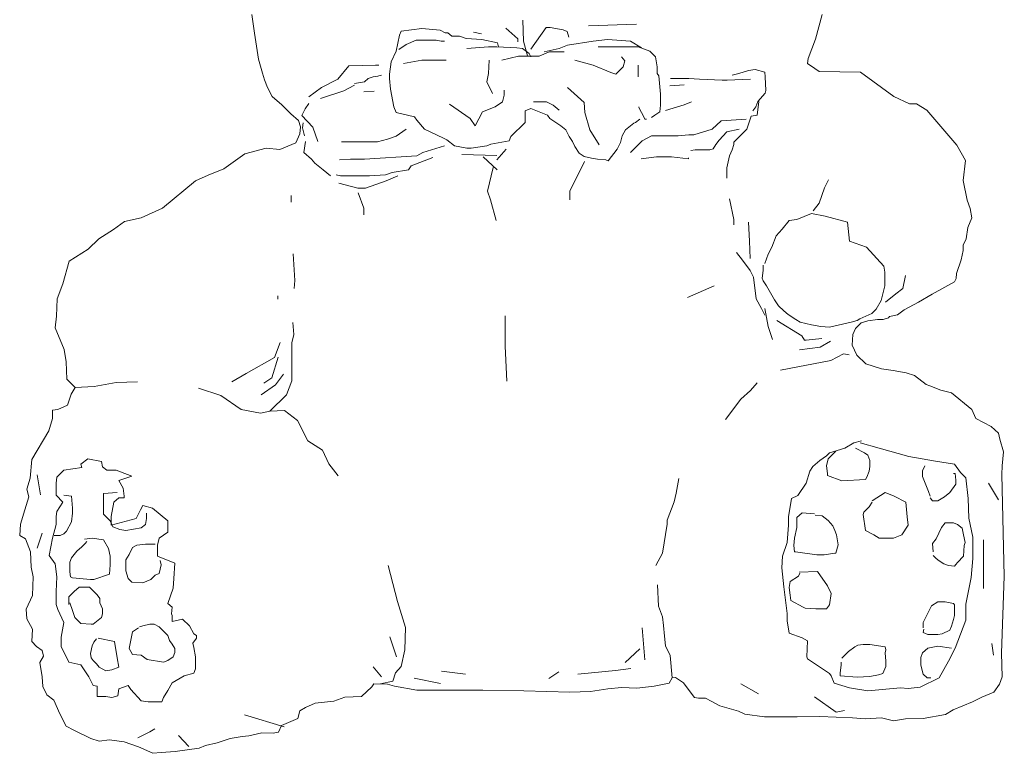
# Model space of a CAD drawing. Units: inches. Extents: x 638 to 1303, y 1 to 699.
# Tile 16 of 21: x 945 to 963, y 577 to 591. Entities that reach past the tile are written whole.
import ezdxf

# ---------------------------------------------------------------- set-up
doc = ezdxf.new("R2010")
doc.units = ezdxf.units.IN
doc.header["$MEASUREMENT"] = 0
doc.layers.add('A-FURN-ACCS', color=8, linetype='Continuous', lineweight=13)

msp = doc.modelspace()

# ---------------------------------------------------------------- linework, layer by layer
at = {"layer": 'A-FURN-ACCS'}
for p, q in [((949.14989, 590.79266), (949.20169, 590.44764)), ((959.42362, 590.34166), (959.54608, 590.79084)), ((951.8738, 590.48873), (952.25259, 590.53415)), ((952.25259, 590.53415), (952.58592, 590.50387)), ((953.77913, 590.53989), (953.99984, 590.34875)), ((954.08812, 590.68691), (954.10284, 590.30464)), ((954.23526, 590.15762), (954.51482, 590.55459)), ((954.51482, 590.55459), (954.58839, 590.55459)), ((954.58839, 590.55459), (954.82381, 590.51048)), ((955.28684, 590.58509), (956.16525, 590.61435)), ((949.20169, 590.44764), (949.27456, 589.97731)), ((951.7829, 590.12537), (951.84351, 590.41303)), ((951.84351, 590.41303), (951.8738, 590.48873)), ((952.58592, 590.50387), (952.67683, 590.45845)), ((952.67683, 590.45845), (952.72227, 590.45845)), ((952.72227, 590.45845), (952.79803, 590.39789)), ((952.79803, 590.39789), (952.93439, 590.39789)), ((952.93439, 590.39789), (953.05561, 590.35247)), ((953.05561, 590.35247), (953.34348, 590.33733)), ((953.19059, 590.46637), (953.33772, 590.43697)), ((953.99984, 590.34875), (953.99984, 590.28994)), ((954.82381, 590.51048), (954.89738, 590.48107)), ((954.89738, 590.48107), (954.92681, 590.37816)), ((951.82835, 590.15565), (951.96471, 590.24649)), ((951.96471, 590.24649), (952.14653, 590.32219)), ((952.14653, 590.32219), (952.51016, 590.32219)), ((952.51016, 590.32219), (952.60107, 590.30705)), ((952.60107, 590.30705), (952.66167, 590.30705)), ((953.07076, 590.17079), (953.46469, 590.20107)), ((953.34348, 590.33733), (953.63136, 590.27677)), ((953.46469, 590.20107), (953.61621, 590.20107)), ((953.61621, 590.20107), (953.97984, 590.18593)), ((953.63136, 590.27677), (953.6465, 590.20107)), ((953.97984, 590.18593), (954.0859, 590.17079)), ((954.0859, 590.17079), (954.2071, 590.07995)), ((954.10284, 590.30464), (954.17641, 590.04)), ((954.47983, 590.11023), (954.75255, 590.17079)), ((954.75255, 590.17079), (954.90406, 590.23135)), ((954.90406, 590.23135), (955.37375, 590.30705)), ((955.37375, 590.30705), (955.63132, 590.33733)), ((955.46466, 590.20107), (956.19192, 590.20107)), ((955.63132, 590.33733), (956.05556, 590.30705)), ((956.05556, 590.30705), (956.25253, 590.18593)), ((956.19192, 590.20107), (956.40404, 590.12537)), ((959.29283, 589.9888), (959.42362, 590.34166)), ((951.69199, 589.92855), (951.7829, 590.12537)), ((953.70711, 589.95883), (954.01014, 590.03453)), ((954.01014, 590.03453), (954.38892, 590.03453)), ((954.2071, 590.07995), (954.2374, 590.01939)), ((954.38892, 590.03453), (954.57073, 590.11023)), ((954.57073, 590.11023), (954.84346, 590.11023)), ((955.9495, 589.94369), (955.8889, 590.01939)), ((956.40404, 590.12537), (956.5101, 590.01939)), ((956.5101, 590.01939), (956.5404, 589.83771)), ((959.27975, 589.89732), (959.29283, 589.9888)), ((949.27456, 589.97731), (949.30982, 589.84812)), ((949.30982, 589.84812), (949.34508, 589.71893)), ((950.72231, 589.61062), (950.91928, 589.85285)), ((950.91928, 589.85285), (951.40411, 589.86799)), ((951.40411, 589.86799), (951.46472, 589.86799)), ((951.66169, 589.70145), (951.69199, 589.92855)), ((951.91926, 589.89827), (952.25259, 589.95883)), ((952.25259, 589.95883), (952.38895, 589.95883)), ((952.38895, 589.95883), (952.61622, 589.95883)), ((952.61622, 589.95883), (952.69198, 589.95883)), ((953.47984, 589.95883), (953.46469, 589.71659)), ((955.04042, 589.95883), (955.37375, 589.86799)), ((955.37375, 589.86799), (955.69193, 589.73173)), ((955.78284, 589.70145), (955.9192, 589.83771)), ((955.9192, 589.83771), (955.9495, 589.94369)), ((956.19192, 589.86799), (956.19192, 589.65603)), ((956.5404, 589.83771), (956.5404, 589.71659)), ((959.41054, 589.80584), (959.27975, 589.89732)), ((959.48901, 589.75356), (959.41054, 589.80584)), ((949.34508, 589.71893), (949.38034, 589.60149)), ((951.2085, 589.56653), (951.27306, 589.62746)), ((951.27306, 589.62746), (951.36274, 589.65255)), ((951.36274, 589.65255), (951.44882, 589.66689)), ((951.44882, 589.66689), (951.46676, 589.67047)), ((951.46676, 589.67047), (951.51338, 589.68839)), ((951.66169, 589.62575), (951.66169, 589.70145)), ((951.67684, 589.42893), (951.66169, 589.62575)), ((953.46469, 589.71659), (953.43439, 589.56519)), ((955.69193, 589.73173), (955.78284, 589.70145)), ((956.5404, 589.71659), (956.5707, 589.67117)), ((956.5707, 589.67117), (956.60101, 589.3381)), ((956.78282, 589.62575), (957.11615, 589.62575)), ((957.11615, 589.62575), (957.31312, 589.61062)), ((957.90322, 589.6858), (958.02658, 589.71661)), ((958.02658, 589.71661), (958.20132, 589.76797)), ((958.20132, 589.76797), (958.32467, 589.78852)), ((958.32467, 589.78852), (958.49942, 589.73716)), ((958.49942, 589.73716), (958.5097, 589.65499)), ((958.5097, 589.65499), (958.51998, 589.40847)), ((960.24757, 589.74049), (959.48901, 589.75356)), ((960.84919, 589.29615), (960.24757, 589.74049)), ((949.38034, 589.60149), (949.4391, 589.46056)), ((949.4391, 589.46056), (949.52138, 589.29614)), ((950.19201, 589.29267), (950.41928, 589.45922)), ((950.41928, 589.45922), (950.72231, 589.61062)), ((950.82837, 589.39866), (951.02533, 589.50463)), ((951.02556, 589.53427), (951.2085, 589.56653)), ((953.43439, 589.56519), (953.54045, 589.35323)), ((954.90406, 589.45922), (955.20709, 589.1867)), ((956.77251, 589.49064), (957.02949, 589.51119)), ((957.31312, 589.61062), (957.7222, 589.59547)), ((957.7222, 589.59547), (957.81311, 589.59547)), ((957.81311, 589.59547), (958.23734, 589.61062)), ((949.52138, 589.29614), (949.69767, 589.14347)), ((950.40413, 589.2624), (950.82837, 589.39866)), ((951.19173, 589.38237), (951.38125, 589.39351)), ((951.73744, 589.111), (951.67684, 589.42893)), ((953.72226, 589.20184), (953.75256, 589.32296)), ((953.75256, 589.32296), (953.75256, 589.4138)), ((956.60101, 589.3381), (956.60101, 589.14128)), ((958.5097, 589.35711), (958.37606, 589.20304)), ((958.51998, 589.40847), (958.5097, 589.35711)), ((961.13692, 589.16547), (960.84919, 589.29615)), ((949.69767, 589.14347), (949.86221, 588.97905)), ((950.18839, 589.17071), (950.1215, 589.07045)), ((951.7829, 589.00502), (951.73744, 589.111)), ((952.75258, 589.15642), (953.13136, 588.89904)), ((953.35863, 589.02016), (953.5859, 589.111)), ((953.5859, 589.111), (953.72226, 589.20184)), ((954.28286, 589.20184), (954.52528, 589.20184)), ((954.52528, 589.20184), (954.64649, 589.14128)), ((954.64649, 589.14128), (954.75255, 589.05044)), ((955.20709, 589.1867), (955.22224, 589.00502)), ((956.20707, 589.09586), (956.20707, 589.111)), ((956.25253, 589.00502), (956.20707, 589.09586)), ((956.60101, 589.14128), (956.58586, 589.02016)), ((956.69168, 589.0428), (957.03133, 589.14723)), ((957.03133, 589.14723), (957.16197, 589.19944)), ((958.33495, 589.11059), (958.28356, 589.0387)), ((958.37606, 589.20304), (958.33495, 589.11059)), ((958.39184, 589.20497), (958.36043, 588.95382)), ((961.2677, 589.16547), (961.13692, 589.16547)), ((961.4508, 589.04785), (961.2677, 589.16547)), ((949.86221, 588.97905), (950.00324, 588.86161)), ((950.1215, 589.07045), (950.06575, 588.94792)), ((950.06575, 588.94792), (950.26642, 588.73626)), ((952.11623, 588.92932), (951.7829, 589.00502)), ((952.16168, 588.86876), (952.11623, 588.92932)), ((953.22227, 588.76278), (953.35863, 589.02016)), ((954.2374, 589.08072), (954.13134, 589.0353)), ((954.13134, 589.0353), (954.13134, 588.91418)), ((954.13134, 588.91418), (954.13134, 588.82334)), ((954.54043, 588.9596), (954.2374, 589.08072)), ((954.58588, 588.89904), (954.54043, 588.9596)), ((955.22224, 589.00502), (955.31315, 588.68708)), ((956.29798, 588.92932), (956.25253, 589.00502)), ((956.31313, 588.8839), (956.29798, 588.92932)), ((956.49495, 588.9596), (956.43434, 588.91418)), ((956.58586, 589.02016), (956.49495, 588.9596)), ((958.25047, 588.93813), (958.17192, 588.70267)), ((958.36043, 588.95382), (958.25047, 588.93813)), ((962.00011, 588.40748), (961.4508, 589.04785)), ((950.00324, 588.86161), (950.03851, 588.74417)), ((950.03851, 588.74417), (950.02675, 588.61498)), ((950.08805, 588.81424), (950.0769, 588.72511)), ((950.26642, 588.73626), (950.35561, 588.48004)), ((952.29804, 588.70222), (952.16168, 588.86876)), ((953.13136, 588.89904), (953.22227, 588.76278)), ((954.13134, 588.82334), (953.87378, 588.56596)), ((954.78285, 588.76278), (954.58588, 588.89904)), ((954.87376, 588.68708), (954.78285, 588.76278)), ((956.11617, 588.8082), (955.96465, 588.68708)), ((956.14647, 588.82334), (956.11617, 588.8082)), ((956.22223, 588.8839), (956.14647, 588.82334)), ((956.34344, 588.8839), (956.31313, 588.8839)), ((957.54039, 588.70222), (957.70705, 588.85362)), ((957.70705, 588.85362), (958.16159, 588.8839)), ((950.02675, 588.61498), (949.95623, 588.45056)), ((950.0769, 588.72511), (950.11035, 588.5803)), ((951.62302, 588.52065), (951.77978, 588.57286)), ((951.77978, 588.57286), (951.96268, 588.7034)), ((952.64652, 588.53568), (952.29804, 588.70222)), ((953.87378, 588.56596), (953.84347, 588.49026)), ((954.93437, 588.56596), (954.87376, 588.68708)), ((954.99497, 588.47512), (954.93437, 588.56596)), ((955.31315, 588.68708), (955.47981, 588.41456)), ((955.90404, 588.5811), (955.87375, 588.45998)), ((955.96465, 588.68708), (955.90404, 588.5811)), ((956.26768, 588.49026), (956.43434, 588.5811)), ((956.43434, 588.5811), (956.91918, 588.5811)), ((956.91918, 588.5811), (957.11615, 588.59624)), ((957.11615, 588.59624), (957.20706, 588.59624)), ((957.20706, 588.59624), (957.54039, 588.70222)), ((957.81063, 588.65558), (957.66925, 588.49862)), ((958.03054, 588.70267), (957.81063, 588.65558)), ((958.17192, 588.70267), (957.93629, 588.46722)), ((949.95623, 588.45056), (949.66241, 588.33312)), ((950.13141, 588.47512), (950.1011, 588.2783)), ((950.78695, 588.46843), (951.44013, 588.46843)), ((951.44013, 588.46843), (951.62302, 588.52065)), ((952.66167, 588.39942), (952.26774, 588.2783)), ((952.70713, 588.5054), (952.64652, 588.53568)), ((952.84349, 588.39942), (952.70713, 588.5054)), ((953.07076, 588.354), (952.84349, 588.39942)), ((953.43439, 588.39942), (953.14652, 588.354)), ((953.51015, 588.4297), (953.43439, 588.39942)), ((953.84347, 588.49026), (953.51015, 588.4297)), ((955.04042, 588.38428), (954.99497, 588.47512)), ((955.11618, 588.26316), (955.04042, 588.38428)), ((955.87375, 588.45998), (955.81314, 588.33886)), ((956.05556, 588.2783), (956.26768, 588.49026)), ((957.60641, 588.42013), (957.55929, 588.34165)), ((957.66925, 588.49862), (957.60641, 588.42013)), ((957.93629, 588.42013), (957.90488, 588.32595)), ((957.93629, 588.46722), (957.93629, 588.42013)), ((962.15705, 588.13303), (962.00011, 588.40748)), ((949.02775, 588.25091), (948.6399, 587.98079)), ((949.4156, 588.35661), (949.02775, 588.25091)), ((949.66241, 588.33312), (949.4156, 588.35661)), ((950.1011, 588.2783), (950.23747, 588.15718)), ((952.16168, 588.21774), (951.20715, 588.15718)), ((952.26774, 588.2783), (952.16168, 588.21774)), ((952.98128, 588.24184), (953.61533, 588.22036)), ((953.14652, 588.354), (953.07076, 588.354)), ((953.36816, 588.19888), (953.62608, 587.96263)), ((953.61533, 588.14519), (953.78729, 588.33849)), ((955.20709, 588.2026), (955.11618, 588.26316)), ((955.34345, 588.17232), (955.20709, 588.2026)), ((955.81314, 588.33886), (955.64648, 588.1269)), ((956.24855, 588.16053), (956.52467, 588.19502)), ((956.52467, 588.19502), (956.80081, 588.19502)), ((956.80081, 588.19502), (957.11145, 588.16053)), ((957.22941, 588.32595), (957.15086, 588.31025)), ((957.49645, 588.32595), (957.22941, 588.32595)), ((957.55929, 588.34165), (957.49645, 588.32595)), ((957.85775, 588.21608), (957.81063, 587.99632)), ((957.90488, 588.32595), (957.85775, 588.21608)), ((950.23747, 588.15718), (950.29807, 588.08148)), ((950.29807, 588.08148), (950.44959, 587.96036)), ((950.94957, 588.15718), (950.75261, 588.14204)), ((951.20715, 588.15718), (950.94957, 588.15718)), ((952.05562, 588.03606), (952.01017, 587.96036)), ((952.44955, 588.18746), (952.05562, 588.03606)), ((955.21288, 588.11011), (954.94507, 587.5749)), ((955.44951, 588.15718), (955.34345, 588.17232)), ((955.60102, 588.14204), (955.44951, 588.15718)), ((955.64648, 588.1269), (955.60102, 588.14204)), ((957.11145, 588.16053), (957.11145, 588.17778)), ((962.11781, 587.7671), (962.15705, 588.13303)), ((948.35783, 587.86335), (948.12277, 587.75766)), ((948.6399, 587.98079), (948.35783, 587.86335)), ((950.44959, 587.96036), (950.58594, 587.85438)), ((950.76776, 587.85438), (950.692, 587.86952)), ((951.29806, 587.85438), (950.76776, 587.85438)), ((951.58593, 587.86952), (951.29806, 587.85438)), ((951.70714, 587.91494), (951.58593, 587.86952)), ((951.60108, 587.76354), (951.8132, 587.85438)), ((952.01017, 587.96036), (951.70714, 587.91494)), ((953.5525, 588.00307), (953.44538, 587.5749)), ((957.81063, 587.99632), (957.81063, 587.80796)), ((948.12277, 587.75766), (947.52337, 587.2644)), ((950.73746, 587.71812), (951.08594, 587.62728)), ((951.2223, 587.62728), (951.60108, 587.76354)), ((959.66424, 587.77656), (959.5857, 587.63529)), ((962.18884, 587.41007), (962.11781, 587.7671)), ((949.87061, 587.49189), (949.87061, 587.3701)), ((951.08594, 587.62728), (951.2223, 587.62728)), ((951.08837, 587.53971), (951.19192, 587.26378)), ((953.44538, 587.5749), (953.49894, 587.41434)), ((954.94507, 587.5749), (954.94507, 587.41434)), ((959.5857, 587.63529), (959.49144, 587.35275)), ((953.49894, 587.41434), (953.60607, 587.0397)), ((957.85775, 587.43123), (957.93629, 587.05451)), ((959.49144, 587.35275), (959.38149, 587.21148)), ((962.2442, 587.25794), (962.18884, 587.41007)), ((947.52337, 587.2644), (947.13552, 587.08824)), ((951.19192, 587.26378), (951.19192, 587.14306)), ((959.08302, 587.05451), (959.35007, 587.16439)), ((959.35007, 587.16439), (959.6014, 587.1173)), ((959.6014, 587.1173), (960.00983, 587.00742)), ((962.27188, 587.08507), (962.2442, 587.25794)), ((946.82995, 587.01777), (946.63014, 586.87684)), ((947.13552, 587.08824), (946.82995, 587.01777)), ((957.93629, 587.05451), (957.93629, 586.96033)), ((958.20334, 587.00742), (958.21905, 586.66209)), ((958.81597, 586.88184), (958.94165, 587.03881)), ((958.94165, 587.03881), (959.08302, 587.05451)), ((960.00983, 587.00742), (960.04124, 586.66209)), ((962.20268, 586.9122), (962.27188, 587.08507)), ((946.63014, 586.87684), (946.36692, 586.7061)), ((958.62747, 586.55221), (958.70601, 586.75627)), ((958.70601, 586.75627), (958.81597, 586.88184)), ((962.16808, 586.70477), (962.20268, 586.9122)), ((946.36692, 586.7061), (946.16711, 586.51819)), ((958.21905, 586.66209), (958.23476, 586.34815)), ((960.04124, 586.66209), (960.35542, 586.55221)), ((962.11272, 586.58721), (962.16808, 586.70477)), ((962.11272, 586.49041), (962.11272, 586.58721)), ((946.16711, 586.51819), (945.82628, 586.29505)), ((949.90596, 586.42933), (949.93844, 585.94243)), ((957.98342, 586.45803), (958.09338, 586.31676)), ((958.50181, 586.25397), (958.56464, 586.42664)), ((958.56464, 586.42664), (958.62747, 586.55221)), ((960.35542, 586.55221), (960.66959, 586.20688)), ((962.07812, 586.32445), (962.11272, 586.49041)), ((945.82628, 586.29505), (945.70875, 585.88401)), ((958.09338, 586.31676), (958.23476, 586.1284)), ((958.47038, 586.1284), (958.47038, 586.22258)), ((961.99508, 586.07552), (962.07812, 586.32445)), ((958.23476, 586.1284), (958.29759, 586.00282)), ((958.45468, 585.98713), (958.47038, 586.1284)), ((960.66959, 586.20688), (960.6853, 586.097)), ((960.6853, 586.097), (960.6853, 585.84586)), ((961.98816, 585.97872), (961.99508, 586.07552)), ((945.70875, 585.88401), (945.60297, 585.61389)), ((949.93844, 585.94243), (949.9222, 585.79636)), ((958.29759, 586.00282), (958.34472, 585.6104)), ((958.47038, 585.94004), (958.45468, 585.98713)), ((958.53322, 585.84586), (958.47038, 585.94004)), ((961.0623, 586.03422), (961.01518, 585.79876)), ((961.55004, 585.69846), (961.96048, 585.9234)), ((961.96048, 585.9234), (961.98816, 585.97872)), ((957.57905, 585.84784), (957.09156, 585.63472)), ((958.6746, 585.59471), (958.53322, 585.84586)), ((960.6853, 585.84586), (960.62246, 585.57901)), ((960.88951, 585.70458), (960.70101, 585.54762)), ((961.01518, 585.79876), (960.88951, 585.70458)), ((961.30092, 585.55325), (961.55004, 585.69846)), ((945.60297, 585.61389), (945.59122, 585.2968)), ((949.62687, 585.66517), (949.62687, 585.60428)), ((958.34472, 585.6104), (958.43897, 585.43774)), ((958.75314, 585.48483), (958.6746, 585.59471)), ((960.62246, 585.57901), (960.52821, 585.42204)), ((961.03796, 585.40804), (961.30092, 585.55325)), ((958.43897, 585.43774), (958.50181, 585.31216)), ((958.50181, 585.43774), (958.56464, 585.1081)), ((958.84739, 585.39065), (958.75314, 585.48483)), ((958.92593, 585.32786), (958.84739, 585.39065)), ((959.06731, 585.23368), (958.92593, 585.32786)), ((960.44967, 585.34356), (960.22975, 585.24938)), ((960.52821, 585.42204), (960.44967, 585.34356)), ((960.92032, 585.31815), (961.03796, 585.40804)), ((945.59122, 585.2968), (945.56771, 585.0854)), ((949.91721, 584.95945), (949.90037, 585.17828)), ((953.77053, 585.29983), (953.77053, 584.75181)), ((958.72172, 585.21798), (959.17727, 584.93544)), ((959.14586, 585.18659), (959.06731, 585.23368)), ((959.35007, 585.1395), (959.14586, 585.18659)), ((960.07266, 585.18659), (959.67995, 585.09241)), ((960.18262, 585.21798), (960.07266, 585.18659)), ((960.15222, 585.06922), (960.25601, 585.17294)), ((960.22975, 585.24938), (960.18262, 585.21798)), ((960.25601, 585.17294), (960.38057, 585.20752)), ((960.38057, 585.20752), (960.55357, 585.23517)), ((960.55357, 585.23517), (960.65737, 585.23517)), ((960.65737, 585.23517), (960.75424, 585.26283)), ((960.75424, 585.26283), (960.77501, 585.29049)), ((960.77501, 585.29049), (960.92032, 585.31815)), ((945.56771, 585.0854), (945.73225, 584.6861)), ((958.56464, 585.1081), (958.64318, 584.87265)), ((959.52286, 585.1081), (959.35007, 585.1395)), ((959.67995, 585.09241), (959.52286, 585.1081)), ((960.10377, 584.95859), (960.15222, 585.06922)), ((949.67082, 584.81513), (949.56443, 584.54176)), ((949.88352, 584.80795), (949.91721, 584.95945)), ((949.88352, 584.40396), (949.88352, 584.80795)), ((959.17727, 584.93544), (959.2244, 584.85695)), ((959.2244, 584.85695), (959.25581, 584.85695)), ((959.25581, 584.85695), (959.53857, 584.88835)), ((959.50715, 584.73138), (959.69565, 584.84126)), ((960.08993, 584.76498), (960.10377, 584.95859)), ((945.73225, 584.6861), (945.76751, 584.46296)), ((953.77053, 584.75181), (953.801, 584.11246)), ((959.13015, 584.68429), (959.50715, 584.73138)), ((959.70471, 584.48715), (959.93399, 584.61052)), ((959.93399, 584.61052), (960.03981, 584.5929)), ((960.1799, 584.58519), (960.08993, 584.76498)), ((945.76751, 584.46296), (945.77926, 584.14587)), ((949.56443, 584.54176), (949.04768, 584.25321)), ((949.62984, 584.54666), (949.51615, 584.17338)), ((958.78756, 584.31091), (959.70471, 584.48715)), ((960.33905, 584.42615), (960.1799, 584.58519)), ((960.62969, 584.33626), (960.33905, 584.42615)), ((949.04768, 584.25321), (948.78931, 584.10134)), ((949.88352, 584.25246), (949.88352, 584.40396)), ((949.88352, 584.1178), (949.88352, 584.25246)), ((960.83729, 584.3086), (960.62969, 584.33626)), ((961.07948, 584.2602), (960.83729, 584.3086)), ((961.23172, 584.2118), (961.07948, 584.2602)), ((945.77926, 584.14587), (945.93205, 583.99319)), ((946.27853, 584.0168), (946.68283, 584.08413)), ((946.68283, 584.08413), (947.07028, 584.10097)), ((949.51615, 584.17338), (949.36997, 584.076)), ((949.72729, 584.2383), (949.58111, 584.04354)), ((949.78245, 583.8653), (949.88352, 584.1178)), ((958.24081, 583.9408), (958.36426, 584.0818)), ((961.43931, 584.05276), (961.23172, 584.2118)), ((945.93205, 583.99319), (945.86154, 583.87576)), ((945.93205, 583.99319), (946.27853, 584.0168)), ((948.18211, 583.98313), (948.5864, 583.84847)), ((949.58111, 584.04354), (949.32124, 583.86501)), ((958.06443, 583.78218), (958.24081, 583.9408)), ((961.50851, 584.0251), (961.43931, 584.05276)), ((961.70919, 583.94904), (961.50851, 584.0251)), ((961.90295, 583.90064), (961.70919, 583.94904)), ((962.27066, 583.59232), (961.90295, 583.90064)), ((945.86154, 583.87576), (945.79102, 583.6761)), ((948.5864, 583.84847), (948.95701, 583.59597)), ((949.47922, 583.5623), (949.78245, 583.8653)), ((957.78223, 583.41208), (958.06443, 583.78218)), ((945.61472, 583.59389), (945.5207, 583.58215)), ((945.5207, 583.58215), (945.5207, 583.42947)), ((945.79102, 583.6761), (945.61472, 583.59389)), ((948.95701, 583.59597), (949.31077, 583.52864)), ((949.31077, 583.52864), (949.47922, 583.5623)), ((949.47922, 583.5623), (949.74876, 583.57914)), ((949.74876, 583.57914), (949.9846, 583.39397)), ((962.34678, 583.43329), (962.27066, 583.59232)), ((945.5207, 583.42947), (945.45018, 583.20634)), ((949.9846, 583.39397), (950.1699, 583.02364)), ((962.62358, 583.28808), (962.34678, 583.43329)), ((945.45018, 583.20634), (945.14507, 582.68286)), ((962.76198, 583.16361), (962.62358, 583.28808)), ((950.1699, 583.02364), (950.43943, 582.85532)), ((960.12587, 582.98582), (960.26454, 583.02739)), ((962.78273, 583.05298), (962.76198, 583.16361)), ((962.85194, 582.82479), (962.78273, 583.05298)), ((950.43943, 582.85532), (950.55735, 582.60282)), ((959.65441, 582.69484), (959.79307, 582.8334)), ((959.68214, 582.80569), (959.95947, 582.88883)), ((959.95947, 582.88883), (960.12587, 582.98582)), ((960.15361, 582.88883), (960.32001, 582.80569)), ((960.23681, 582.98582), (960.58348, 582.88883)), ((960.58348, 582.88883), (961.12428, 582.73641)), ((962.82426, 582.56895), (962.85194, 582.82479)), ((945.14507, 582.68286), (945.10982, 582.34228)), ((946.16406, 582.69357), (946.03854, 582.5995)), ((946.41509, 582.64654), (946.16406, 582.69357)), ((946.43078, 582.55247), (946.41509, 582.64654)), ((959.37707, 582.55627), (959.50187, 582.66713)), ((959.50187, 582.66713), (959.62667, 582.75027)), ((959.62667, 582.75027), (959.68214, 582.80569)), ((959.62667, 582.57013), (959.65441, 582.69484)), ((960.32001, 582.80569), (960.37547, 582.76412)), ((960.37547, 582.76412), (960.41708, 582.66713)), ((960.41708, 582.66713), (960.41708, 582.55627)), ((961.12428, 582.73641), (961.60962, 582.65327)), ((961.60962, 582.65327), (961.95629, 582.59785)), ((945.72476, 582.48976), (945.59924, 582.36434)), ((946.05423, 582.53679), (945.72476, 582.48976)), ((946.03854, 582.5995), (946.05423, 582.53679)), ((946.50923, 582.48976), (946.43078, 582.55247)), ((946.68181, 582.48976), (946.50923, 582.48976)), ((946.76026, 582.4584), (946.68181, 582.48976)), ((946.96423, 582.38002), (946.76026, 582.4584)), ((950.55735, 582.60282), (950.72581, 582.38399)), ((959.25227, 582.25144), (959.3216, 582.47314)), ((959.3216, 582.47314), (959.37707, 582.55627)), ((959.64054, 582.43157), (959.62667, 582.57013)), ((960.40321, 582.47314), (960.36161, 582.36229)), ((960.41708, 582.55627), (960.40321, 582.47314)), ((961.40162, 582.52856), (961.37388, 582.48699)), ((961.37388, 582.48699), (961.37388, 582.37614)), ((961.41548, 582.57013), (961.40162, 582.52856)), ((961.95629, 582.59785), (962.06722, 582.44542)), ((962.81733, 582.40991), (962.82426, 582.56895)), ((945.10982, 582.34228), (945.05105, 582.14263)), ((945.23946, 582.40752), (945.3004, 582.04218)), ((945.59924, 582.36434), (945.58355, 582.25459)), ((946.72888, 582.30163), (946.96423, 582.38002)), ((946.80733, 582.16053), (946.72888, 582.30163)), ((956.88272, 582.07264), (956.93564, 582.33701)), ((959.64054, 582.39), (959.64054, 582.43157)), ((959.90401, 582.293), (959.64054, 582.39)), ((960.33387, 582.32072), (959.90401, 582.293)), ((960.36161, 582.36229), (960.33387, 582.32072)), ((961.37388, 582.37614), (961.48482, 582.09901)), ((961.97015, 582.43157), (961.94242, 582.43157)), ((961.98402, 582.30686), (961.97015, 582.43157)), ((961.98402, 582.23758), (961.98402, 582.30686)), ((962.06722, 582.44542), (962.16429, 582.34843)), ((962.16429, 582.34843), (962.20589, 581.97431)), ((962.86534, 580.55802), (962.81733, 582.40991)), ((945.05105, 582.14263), (945.08631, 582.0017)), ((945.58355, 582.25459), (945.58355, 582.0351)), ((946.82302, 582.01943), (946.80733, 582.16053)), ((959.09973, 582.02973), (959.25227, 582.25144)), ((961.48482, 582.09901), (961.51255, 582.01588)), ((961.87309, 582.08516), (961.98402, 582.23758)), ((962.57582, 582.2553), (962.75863, 581.95085)), ((945.08631, 582.0017), (945.01579, 581.76682)), ((945.58355, 582.0351), (945.70907, 581.90968)), ((945.72476, 582.0351), (945.86596, 582.01943)), ((945.86596, 582.01943), (945.88165, 581.79994)), ((946.6975, 582.08214), (946.44647, 582.06646)), ((946.44647, 582.06646), (946.44647, 581.83129)), ((946.63475, 581.90968), (946.72888, 581.98807)), ((946.72888, 581.98807), (946.82302, 581.98807)), ((946.82302, 581.98807), (946.82302, 582.01943)), ((956.72399, 581.57917), (956.84745, 581.91403)), ((956.84745, 581.91403), (956.88272, 582.07264)), ((958.93333, 581.64175), (958.9888, 581.97431)), ((958.9888, 581.97431), (959.09973, 582.02973)), ((960.45868, 581.93274), (960.69441, 582.08516)), ((960.69441, 582.08516), (960.86082, 582.01588)), ((960.86082, 582.01588), (961.06882, 581.90503)), ((961.51255, 581.98816), (961.55415, 581.93274)), ((961.55415, 581.93274), (961.65122, 581.93274)), ((961.65122, 581.93274), (961.77602, 582.00202)), ((961.77602, 582.00202), (961.87309, 582.08516)), ((962.20589, 581.97431), (962.21976, 581.61404)), ((945.01579, 581.76682), (944.93352, 581.50845)), ((945.59924, 581.73723), (945.58355, 581.64316)), ((945.70907, 581.90968), (945.59924, 581.73723)), ((945.88165, 581.79994), (945.88165, 581.70587)), ((946.44647, 581.83129), (946.44647, 581.69019)), ((946.58768, 581.64316), (946.63475, 581.90968)), ((947.12112, 581.76858), (947.04267, 581.61181)), ((947.16819, 581.84697), (947.12112, 581.76858)), ((947.34077, 581.79994), (947.16819, 581.84697)), ((947.62319, 581.56477), (947.34077, 581.79994)), ((960.30614, 581.72489), (960.40321, 581.82189)), ((960.40321, 581.82189), (960.45868, 581.90503)), ((961.06882, 581.90503), (961.09655, 581.64175)), ((945.58355, 581.64316), (945.58355, 581.50206)), ((945.88165, 581.70587), (945.86596, 581.5491)), ((946.44647, 581.69019), (946.57199, 581.56477)), ((946.57199, 581.56477), (946.61906, 581.45503)), ((946.58768, 581.48638), (946.58768, 581.64316)), ((947.04267, 581.61181), (946.58768, 581.48638)), ((947.21526, 581.50206), (947.23095, 581.61181)), ((947.23095, 581.61181), (947.23095, 581.70587)), ((947.62319, 581.36096), (947.62319, 581.56477)), ((956.72399, 581.50867), (956.72399, 581.57917)), ((958.93333, 581.48933), (958.93333, 581.64175)), ((959.08587, 581.6279), (959.18294, 581.71104)), ((959.08587, 581.44777), (959.08587, 581.6279)), ((959.18294, 581.71104), (959.4048, 581.69718)), ((959.41867, 581.66947), (959.54347, 581.65561)), ((959.54347, 581.65561), (959.65441, 581.57247)), ((959.65441, 581.57247), (959.73761, 581.47548)), ((960.29227, 581.68332), (960.30614, 581.72489)), ((960.33387, 581.39234), (960.29227, 581.68332)), ((961.09655, 581.64175), (961.11042, 581.48933)), ((962.21976, 581.61404), (962.28909, 581.26763)), ((944.93352, 581.50845), (944.92177, 581.29705)), ((945.58355, 581.50206), (945.52079, 581.25122)), ((945.77182, 581.37664), (945.72476, 581.32961)), ((945.86596, 581.5491), (945.77182, 581.37664)), ((946.61906, 581.45503), (946.74457, 581.40799)), ((946.74457, 581.40799), (946.8544, 581.39232)), ((946.8544, 581.39232), (947.13681, 581.43935)), ((947.13681, 581.43935), (947.21526, 581.50206)), ((956.6358, 580.97995), (956.72399, 581.50867)), ((958.9056, 581.17064), (958.93333, 581.48933)), ((959.04427, 581.25377), (959.08587, 581.44777)), ((959.73761, 581.47548), (959.77921, 581.39234)), ((959.77921, 581.39234), (959.80694, 581.3092)), ((960.48641, 581.3092), (960.33387, 581.39234)), ((961.11042, 581.48933), (960.99948, 581.3092)), ((961.62349, 581.23992), (961.72055, 581.44777)), ((961.72055, 581.44777), (961.78989, 581.5309)), ((961.78989, 581.5309), (961.94242, 581.5309)), ((961.94242, 581.5309), (962.01175, 581.50319)), ((962.01175, 581.50319), (962.09496, 581.43391)), ((962.09496, 581.43391), (962.12269, 581.3092)), ((944.92177, 581.29705), (945.02754, 581.23833)), ((945.02754, 581.23833), (945.12157, 581.00345)), ((945.23946, 581.06793), (945.33087, 581.34194)), ((945.52079, 581.25122), (945.45804, 580.93766)), ((945.56786, 581.29825), (945.55217, 581.29825)), ((945.66199, 581.29825), (945.56786, 581.29825)), ((945.72476, 581.32961), (945.66199, 581.29825)), ((946.1013, 581.23554), (946.24251, 581.25122)), ((946.24251, 581.25122), (946.44647, 581.21986)), ((946.44647, 581.21986), (946.54061, 581.06308)), ((947.43491, 581.1258), (947.46629, 581.25122)), ((947.46629, 581.25122), (947.62319, 581.36096)), ((959.0304, 581.11521), (959.04427, 581.25377)), ((959.80694, 581.3092), (959.83467, 581.12907)), ((960.58348, 581.25377), (960.48641, 581.3092)), ((960.74988, 581.25377), (960.58348, 581.25377)), ((960.84695, 581.25377), (960.74988, 581.25377)), ((960.99948, 581.3092), (960.84695, 581.25377)), ((961.55415, 581.15678), (961.62349, 581.23992)), ((962.12269, 581.3092), (962.15042, 581.17064)), ((962.28909, 581.26763), (962.28909, 580.87965)), ((962.48442, 581.22016), (962.48442, 581.06793)), ((945.86596, 580.89063), (945.9601, 581.01605)), ((945.9601, 581.01605), (946.05423, 581.09444)), ((946.05423, 581.09444), (946.11699, 581.15715)), ((946.11699, 581.15715), (946.14837, 581.18851)), ((946.54061, 581.06308), (946.57199, 580.92198)), ((946.97992, 581.07876), (946.91715, 580.95334)), ((947.05836, 581.1258), (946.97992, 581.07876)), ((947.21526, 581.14147), (947.05836, 581.1258)), ((947.38784, 581.14147), (947.21526, 581.14147)), ((947.43491, 580.96902), (947.43491, 581.1258)), ((958.8224, 580.92122), (958.9056, 581.17064)), ((959.04427, 581.00436), (959.0304, 581.11521)), ((959.83467, 581.12907), (959.79307, 580.97665)), ((961.56802, 581.00436), (961.55415, 581.15678)), ((962.13656, 581.11521), (962.12269, 580.92122)), ((962.15042, 581.17064), (962.13656, 581.11521)), ((962.48442, 581.06793), (962.48442, 580.33724)), ((945.12157, 581.00345), (945.13332, 580.72159)), ((945.45804, 580.93766), (945.56786, 580.78089)), ((945.83458, 580.81224), (945.86596, 580.89063)), ((946.57199, 580.92198), (946.57199, 580.76521)), ((946.91715, 580.95334), (946.8544, 580.85927)), ((946.8544, 580.85927), (946.8544, 580.65546)), ((947.43491, 580.92198), (947.43491, 580.96902)), ((947.7487, 580.79656), (947.43491, 580.92198)), ((947.49767, 580.76521), (947.48198, 580.8436)), ((956.51234, 580.75083), (956.6358, 580.97995)), ((958.80853, 580.71338), (958.8224, 580.92122)), ((959.05813, 581.00436), (959.04427, 581.00436)), ((959.4464, 580.94893), (959.05813, 581.00436)), ((959.58507, 580.94893), (959.4464, 580.94893)), ((959.77921, 580.97665), (959.58507, 580.94893)), ((959.79307, 580.97665), (959.77921, 580.97665)), ((961.62349, 580.87965), (961.56802, 580.93508)), ((961.67895, 580.83808), (961.62349, 580.87965)), ((961.76215, 580.78266), (961.67895, 580.83808)), ((962.12269, 580.92122), (962.01175, 580.81037)), ((962.28909, 580.87965), (962.26136, 580.53324)), ((945.13332, 580.72159), (945.16858, 580.54543)), ((945.56786, 580.78089), (945.59924, 580.54572)), ((945.83458, 580.63978), (945.83458, 580.81224)), ((946.57199, 580.76521), (946.5563, 580.59275)), ((946.8544, 580.65546), (946.90147, 580.51436)), ((947.46629, 580.60843), (947.49767, 580.76521)), ((947.73301, 580.51436), (947.7487, 580.79656)), ((951.63548, 580.75118), (951.80393, 580.09469)), ((958.85013, 580.36697), (958.80853, 580.71338)), ((961.84535, 580.75495), (961.76215, 580.78266)), ((961.95629, 580.74109), (961.84535, 580.75495)), ((961.98402, 580.7688), (961.95629, 580.74109)), ((962.01175, 580.81037), (961.98402, 580.7688)), ((945.16858, 580.54543), (945.15683, 580.20484)), ((945.59924, 580.54572), (945.58355, 580.2792)), ((945.85027, 580.54572), (945.83458, 580.63978)), ((945.88165, 580.53004), (945.85027, 580.54572)), ((946.21113, 580.49869), (945.88165, 580.53004)), ((946.27389, 580.49869), (946.21113, 580.49869)), ((946.5563, 580.59275), (946.27389, 580.49869)), ((946.90147, 580.51436), (946.96423, 580.45165)), ((947.16819, 580.43597), (947.30939, 580.49869)), ((947.30939, 580.49869), (947.38784, 580.57707)), ((947.38784, 580.57707), (947.46629, 580.60843)), ((947.71732, 580.34191), (947.73301, 580.51436)), ((958.96107, 580.46396), (959.1136, 580.56095)), ((959.1136, 580.56095), (959.14133, 580.61638)), ((959.12747, 580.63024), (959.46027, 580.64409)), ((959.46027, 580.64409), (959.64054, 580.38082)), ((962.26136, 580.53324), (962.16429, 580.04827)), ((962.8169, 579.15433), (962.86534, 580.55802)), ((946.00716, 580.35759), (945.91303, 580.2792)), ((946.02285, 580.35759), (946.00716, 580.35759)), ((946.19544, 580.35759), (946.02285, 580.35759)), ((946.27389, 580.2792), (946.19544, 580.35759)), ((946.96423, 580.45165), (947.16819, 580.43597)), ((947.62319, 580.05971), (947.71732, 580.34191)), ((956.56525, 580.01062), (956.54762, 580.39835)), ((958.9056, 579.88199), (958.85013, 580.36697)), ((958.9472, 580.35311), (958.96107, 580.46396)), ((958.96107, 580.21454), (958.9472, 580.35311)), ((959.64054, 580.38082), (959.70987, 580.24226)), ((945.15683, 580.20484), (945.0393, 579.95822)), ((945.58355, 580.2792), (945.58355, 580.04403)), ((945.91303, 580.2792), (945.81889, 580.18513)), ((945.81889, 580.18513), (945.81889, 580.07539)), ((946.33665, 580.21648), (946.27389, 580.2792)), ((946.38371, 580.15377), (946.33665, 580.21648)), ((946.38371, 580.07539), (946.38371, 580.15377)), ((958.97493, 580.11755), (958.96107, 580.21454)), ((959.1968, 579.99284), (958.97493, 580.11755)), ((959.70987, 580.24226), (959.68214, 580.03441)), ((945.0393, 579.95822), (945.05105, 579.78205)), ((945.58355, 580.04403), (945.61493, 579.94997)), ((945.61493, 579.94997), (945.72476, 579.7148)), ((945.81889, 580.07539), (945.81889, 580.04403)), ((945.83458, 580.07539), (945.88165, 579.93429)), ((946.43078, 579.96564), (946.38371, 580.07539)), ((946.43078, 579.91861), (946.43078, 579.96564)), ((947.70163, 579.997), (947.62319, 580.05971)), ((947.68594, 579.87158), (947.70163, 579.997)), ((951.80393, 580.09469), (951.95555, 579.62336)), ((956.6358, 579.81675), (956.56525, 580.01062)), ((959.2384, 579.97899), (959.1968, 579.99284)), ((959.43254, 579.96513), (959.2384, 579.97899)), ((959.62667, 579.96513), (959.43254, 579.96513)), ((959.68214, 580.03441), (959.62667, 579.96513)), ((961.44322, 579.82657), (961.54028, 580.02056)), ((961.54028, 580.02056), (961.65122, 580.08984)), ((961.65122, 580.08984), (961.78989, 580.08984)), ((961.78989, 580.08984), (961.94242, 580.06213)), ((961.94242, 580.06213), (961.95629, 580.03441)), ((961.95629, 580.03441), (961.95629, 579.84042)), ((962.16429, 580.04827), (962.16429, 579.75728)), ((945.05105, 579.78205), (945.15683, 579.59415)), ((945.88165, 579.93429), (945.92872, 579.80886)), ((945.92872, 579.80886), (946.03854, 579.69912)), ((946.2582, 579.68344), (946.41509, 579.80886)), ((946.41509, 579.80886), (946.43078, 579.87158)), ((946.43078, 579.87158), (946.43078, 579.91861)), ((947.70163, 579.84022), (947.68594, 579.87158)), ((947.70163, 579.73048), (947.70163, 579.84022)), ((947.88991, 579.77751), (947.70163, 579.73048)), ((948.01542, 579.65209), (947.88991, 579.77751)), ((956.65344, 579.65813), (956.6358, 579.81675)), ((958.9056, 579.74343), (958.9056, 579.88199)), ((961.38775, 579.71572), (961.44322, 579.82657)), ((961.94242, 579.77114), (961.90082, 579.64643)), ((961.95629, 579.84042), (961.94242, 579.77114)), ((962.16429, 579.75728), (961.97015, 579.2446)), ((945.15683, 579.59415), (945.14507, 579.37101)), ((945.72476, 579.7148), (945.67768, 579.44828)), ((946.03854, 579.69912), (946.22682, 579.68344)), ((946.22682, 579.68344), (946.2582, 579.68344)), ((947.08974, 579.62073), (946.97992, 579.54234)), ((947.16819, 579.65209), (947.10543, 579.63641)), ((947.2937, 579.68344), (947.16819, 579.65209)), ((947.37215, 579.68344), (947.2937, 579.68344)), ((947.46629, 579.63641), (947.37215, 579.68344)), ((947.54474, 579.55802), (947.46629, 579.63641)), ((948.09387, 579.51099), (948.01542, 579.65209)), ((951.95555, 579.62336), (951.9387, 579.21936)), ((956.26371, 579.61724), (956.31204, 579.03781)), ((956.67108, 579.46427), (956.65344, 579.65813)), ((958.9472, 579.52172), (958.9056, 579.74343)), ((961.38775, 579.61872), (961.38775, 579.71572)), ((961.38775, 579.53558), (961.40162, 579.59101)), ((961.90082, 579.64643), (961.87309, 579.57715)), ((945.67768, 579.44828), (945.67768, 579.27582)), ((946.27389, 579.35421), (946.32095, 579.41692)), ((946.35234, 579.4326), (946.65043, 579.36989)), ((946.97992, 579.54234), (946.91715, 579.24447)), ((947.62319, 579.47963), (947.54474, 579.55802)), ((947.65456, 579.38556), (947.62319, 579.47963)), ((948.07818, 579.33853), (948.14094, 579.4326)), ((948.14094, 579.47963), (948.09387, 579.51099)), ((948.14094, 579.4326), (948.14094, 579.47963)), ((951.66823, 579.45433), (951.7901, 579.08899)), ((956.68872, 579.28803), (956.67108, 579.46427)), ((959.18294, 579.43859), (958.9472, 579.52172)), ((959.28, 579.38316), (959.18294, 579.43859)), ((961.47095, 579.49401), (961.38775, 579.53558)), ((961.52642, 579.49401), (961.47095, 579.49401)), ((961.65122, 579.49401), (961.52642, 579.49401)), ((961.73442, 579.50787), (961.65122, 579.49401)), ((961.87309, 579.57715), (961.73442, 579.50787)), ((945.14507, 579.37101), (945.22735, 579.27705)), ((945.22735, 579.27705), (945.33312, 579.20659)), ((945.67768, 579.27582), (945.81889, 578.99362)), ((946.21113, 579.1504), (946.24251, 579.2915)), ((946.24251, 579.2915), (946.27389, 579.35421)), ((946.65043, 579.36989), (946.6975, 579.07201)), ((946.91715, 579.24447), (946.97992, 579.13472)), ((947.70163, 579.32285), (947.65456, 579.38556)), ((947.7487, 579.24447), (947.70163, 579.32285)), ((947.7487, 579.16608), (947.7487, 579.24447)), ((948.09387, 579.26014), (948.07818, 579.33853)), ((948.12525, 579.08769), (948.09387, 579.26014)), ((951.9387, 579.21936), (951.87132, 578.91637)), ((955.95758, 578.98796), (956.22017, 579.23786)), ((956.7769, 579.11178), (956.68872, 579.28803)), ((959.26614, 579.09218), (959.28, 579.38316)), ((960.02881, 579.18917), (960.13974, 579.27231)), ((960.13974, 579.27231), (960.19521, 579.30002)), ((960.19521, 579.30002), (960.29227, 579.31388)), ((960.29227, 579.31388), (960.37547, 579.31388)), ((960.37547, 579.31388), (960.41708, 579.31388)), ((960.41708, 579.31388), (960.69441, 579.27231)), ((960.69441, 579.27231), (960.70828, 579.21689)), ((961.47095, 579.2446), (961.37388, 579.16146)), ((961.65122, 579.28617), (961.47095, 579.2446)), ((961.90082, 579.2446), (961.65122, 579.28617)), ((961.97015, 579.2446), (961.84535, 579.00904)), ((962.63676, 579.33255), (962.66723, 579.11943)), ((945.35663, 579.10089), (945.28611, 578.98345)), ((945.33312, 579.20659), (945.35663, 579.10089)), ((946.22682, 579.07201), (946.21113, 579.1504)), ((946.2582, 579.02498), (946.22682, 579.07201)), ((946.6975, 579.07201), (946.72888, 578.89956)), ((946.97992, 579.13472), (947.13681, 579.11904)), ((947.13681, 579.11904), (947.24664, 579.04065)), ((947.24664, 579.04065), (947.54474, 578.99362)), ((947.62319, 579.02498), (947.71732, 579.08769)), ((947.71732, 579.08769), (947.7487, 579.16608)), ((948.12525, 578.8682), (948.12525, 579.08769)), ((956.81534, 578.70683), (956.7769, 579.11178)), ((959.28, 579.05061), (959.26614, 579.09218)), ((959.68214, 578.78734), (959.28, 579.05061)), ((959.90401, 579.06446), (960.02881, 579.18917)), ((960.70828, 579.21689), (960.69441, 579.16146)), ((960.69441, 579.16146), (960.70828, 579.00904)), ((961.37388, 579.16146), (961.34615, 579.07832)), ((961.34615, 579.07832), (961.34615, 578.93976)), ((962.82382, 578.72562), (962.8169, 579.15433)), ((945.28611, 578.98345), (945.33312, 578.72508)), ((945.81889, 578.99362), (946.03854, 578.94659)), ((946.03854, 578.94659), (946.17975, 578.7271)), ((946.32095, 578.96227), (946.2582, 579.02498)), ((946.36802, 578.89956), (946.32095, 578.96227)), ((946.49354, 578.83685), (946.36802, 578.89956)), ((946.72888, 578.89956), (946.60337, 578.85252)), ((947.54474, 578.99362), (947.62319, 579.02498)), ((948.09387, 578.78981), (948.12525, 578.8682)), ((951.5159, 578.72365), (951.36355, 578.90632)), ((951.87132, 578.91637), (951.77024, 578.79854)), ((955.78252, 578.83802), (956.05761, 578.87551)), ((959.87627, 578.80119), (959.89014, 578.93976)), ((959.89014, 578.93976), (959.89014, 578.99518)), ((960.70828, 578.91204), (960.65281, 578.78734)), ((960.70828, 579.00904), (960.70828, 578.91204)), ((961.34615, 578.93976), (961.38775, 578.77348)), ((961.84535, 579.00904), (961.67895, 578.7042)), ((945.33312, 578.72508), (945.34488, 578.54891)), ((946.17975, 578.7271), (946.2582, 578.57032)), ((946.60337, 578.85252), (946.49354, 578.83685)), ((947.70163, 578.61735), (947.92128, 578.74278)), ((947.92128, 578.74278), (948.09387, 578.78981)), ((951.77024, 578.79854), (951.71971, 578.64704)), ((952.10806, 578.69982), (952.59127, 578.60324)), ((952.60641, 578.82553), (953.04406, 578.77555)), ((954.74551, 578.81498), (954.5627, 578.6932)), ((955.09478, 578.77555), (955.78252, 578.83802)), ((956.75657, 578.61287), (956.81534, 578.70683)), ((956.81534, 578.70683), (956.87537, 578.71045)), ((956.87537, 578.71045), (957.02069, 578.61365)), ((959.70987, 578.74577), (959.68214, 578.78734)), ((959.76534, 578.6072), (959.70987, 578.74577)), ((959.87627, 578.74577), (959.87627, 578.80119)), ((960.18134, 578.71805), (959.87627, 578.74577)), ((960.41708, 578.73191), (960.18134, 578.71805)), ((960.56961, 578.75963), (960.41708, 578.73191)), ((960.65281, 578.78734), (960.56961, 578.75963)), ((961.67895, 578.7042), (961.33228, 578.53792)), ((961.38775, 578.77348), (961.45708, 578.7042)), ((961.45708, 578.7042), (961.51255, 578.7042)), ((961.51255, 578.7042), (961.52642, 578.7042)), ((962.77538, 578.59424), (962.82382, 578.72562)), ((945.34488, 578.54891), (945.41539, 578.39624)), ((946.2582, 578.57032), (946.33665, 578.55464)), ((946.33665, 578.55464), (946.33665, 578.36651)), ((946.71319, 578.38219), (946.72888, 578.50761)), ((946.72888, 578.50761), (946.90147, 578.57032)), ((946.90147, 578.57032), (946.94853, 578.49193)), ((947.62319, 578.47626), (947.70163, 578.61735)), ((951.15327, 578.36587), (951.34132, 578.54203)), ((951.34132, 578.54203), (951.37658, 578.60075)), ((951.37658, 578.60075), (951.62339, 578.58901)), ((951.71971, 578.64704), (951.49998, 578.59488)), ((951.62339, 578.58901), (951.75267, 578.55378)), ((951.75267, 578.55378), (952.16116, 578.48369)), ((955.32271, 578.4602), (955.64004, 578.50718)), ((955.64004, 578.50718), (955.88685, 578.53067)), ((955.88685, 578.53067), (956.16893, 578.51892)), ((956.16893, 578.51892), (956.48626, 578.55415)), ((956.48626, 578.55415), (956.75657, 578.61287)), ((957.02069, 578.61365), (957.13833, 578.45461)), ((958.06297, 578.59856), (958.38751, 578.41839)), ((960.04267, 578.52407), (959.76534, 578.6072)), ((960.37547, 578.46864), (960.04267, 578.52407)), ((960.97175, 578.52407), (960.37547, 578.46864)), ((961.11042, 578.51021), (960.97175, 578.52407)), ((961.33228, 578.53792), (961.11042, 578.51021)), ((962.67158, 578.44903), (962.77538, 578.59424)), ((945.41539, 578.39624), (945.54467, 578.30229)), ((946.33665, 578.36651), (946.49354, 578.36651)), ((946.49354, 578.36651), (946.60337, 578.35084)), ((946.60337, 578.35084), (946.71319, 578.38219)), ((946.94853, 578.49193), (947.13681, 578.28812)), ((947.51336, 578.27244), (947.54474, 578.35084)), ((947.54474, 578.35084), (947.62319, 578.47626)), ((950.64789, 578.28366), (950.84769, 578.35412)), ((950.84769, 578.35412), (951.15327, 578.36587)), ((952.16116, 578.48369), (952.76056, 578.48369)), ((952.76056, 578.48369), (953.35997, 578.48369)), ((953.35997, 578.48369), (954.11215, 578.47194)), ((954.11215, 578.47194), (954.94662, 578.44846)), ((954.94662, 578.44846), (955.32271, 578.4602)), ((957.13833, 578.45461), (957.22136, 578.35089)), ((957.22136, 578.35089), (957.29056, 578.33706)), ((957.29056, 578.33706), (957.42204, 578.33706)), ((957.42204, 578.33706), (957.53276, 578.27483)), ((959.40713, 578.3583), (959.80322, 578.0843)), ((962.28407, 578.26925), (962.45707, 578.35223)), ((962.45707, 578.35223), (962.67158, 578.44903)), ((945.54467, 578.30229), (945.65288, 578.04878)), ((947.13681, 578.28812), (947.26233, 578.27244)), ((947.26233, 578.27244), (947.51336, 578.27244)), ((950.02499, 578.1075), (950.13076, 578.16622)), ((950.13076, 578.16622), (950.30706, 578.24843)), ((950.30706, 578.24843), (950.64789, 578.28366)), ((957.53276, 578.27483), (957.67808, 578.19877)), ((957.67808, 578.19877), (958.02407, 578.10196)), ((961.93116, 578.12404), (962.28407, 578.26925)), ((945.65288, 578.04878), (945.7704, 577.82564)), ((949.02128, 578.03364), (949.74085, 577.8124)), ((949.6959, 577.83738), (949.98973, 577.96657)), ((949.98973, 577.96657), (950.02499, 578.1075)), ((958.02407, 578.10196), (958.13479, 578.04664)), ((958.13479, 578.04664), (958.49463, 577.99824)), ((958.49463, 577.99824), (959.08974, 577.99824)), ((959.08974, 577.99824), (959.50493, 578.00515)), ((959.50493, 578.00515), (960.09738, 577.97883)), ((959.80322, 578.0843), (959.95556, 578.11474)), ((960.09738, 577.97883), (960.33266, 577.95809)), ((960.33266, 577.95809), (960.63021, 577.97883)), ((960.63021, 577.97883), (960.84473, 577.92351)), ((961.06616, 577.95809), (961.38448, 577.965)), ((961.38448, 577.965), (961.79275, 578.04106)), ((961.79275, 578.04106), (961.93116, 578.12404)), ((945.7704, 577.82564), (945.91144, 577.75517)), ((949.63714, 577.71994), (949.6959, 577.83738)), ((960.84473, 577.92351), (961.06616, 577.95809)), ((945.91144, 577.75517), (946.21702, 577.6025)), ((947.07292, 577.61328), (947.29432, 577.7239)), ((947.29432, 577.7239), (947.38289, 577.77921)), ((947.81463, 577.65753), (948.00282, 577.45842)), ((948.75566, 577.6025), (948.97897, 577.63773)), ((948.97897, 577.63773), (949.0965, 577.64948)), ((949.0965, 577.64948), (949.33156, 577.7082)), ((949.33156, 577.7082), (949.54311, 577.69645)), ((949.54311, 577.69645), (949.63714, 577.71994)), ((946.21702, 577.6025), (946.36981, 577.55552)), ((946.36981, 577.55552), (946.55786, 577.57901)), ((946.55786, 577.57901), (946.82817, 577.54378)), ((946.82817, 577.54378), (947.08674, 577.44982)), ((947.08674, 577.44982), (947.34531, 577.33238)), ((947.75666, 577.36761), (948.19152, 577.42634)), ((948.19152, 577.42634), (948.30905, 577.47331)), ((948.30905, 577.47331), (948.5206, 577.52029)), ((948.5206, 577.52029), (948.75566, 577.6025)), ((947.34531, 577.33238), (947.49809, 577.34413)), ((947.49809, 577.34413), (947.75666, 577.36761))]:
    msp.add_line(p, q, dxfattribs=at)

doc.saveas('drawing.dxf')
